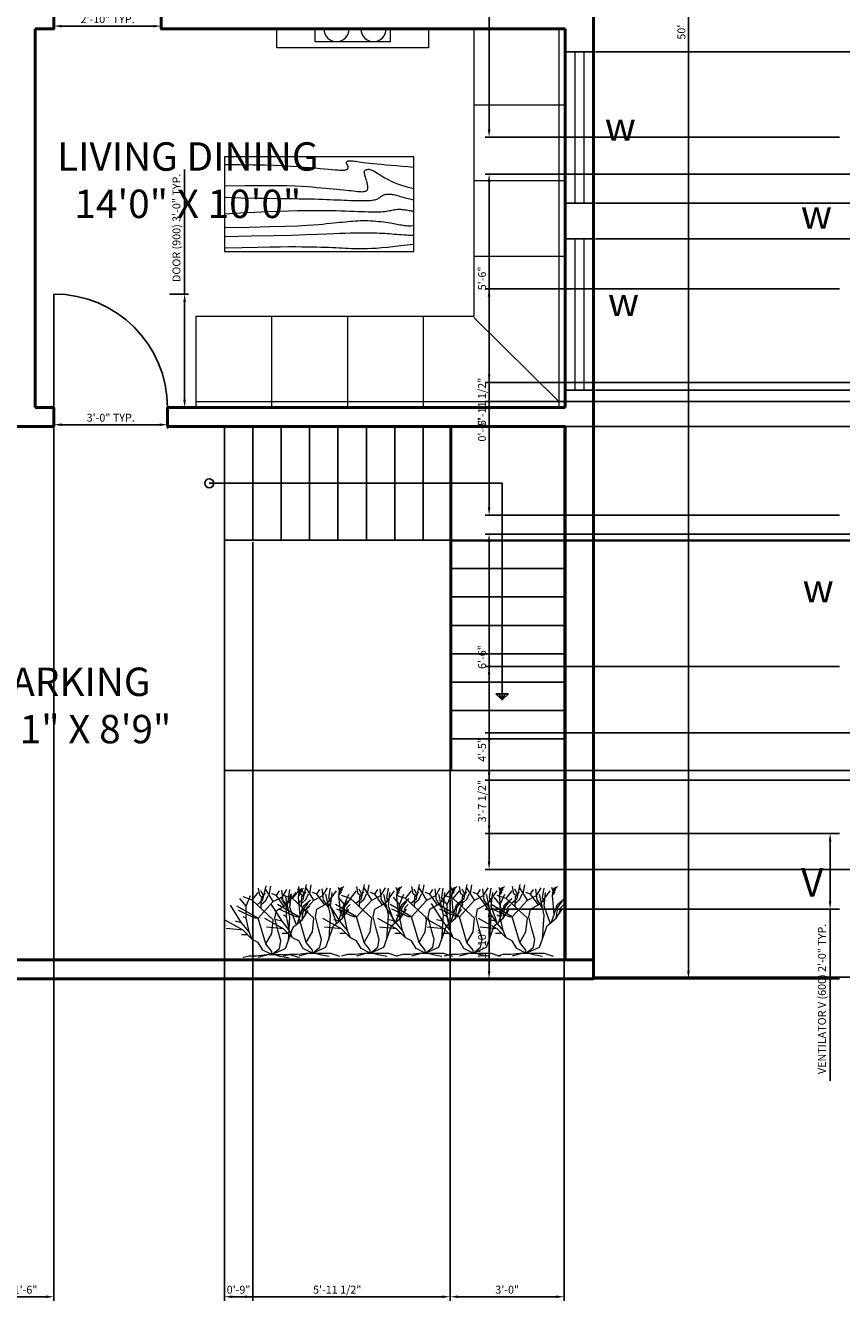
# Model space of a CAD drawing. Units: inches. Extents: x 3688 to 4628, y 1593 to 2337.
# Tile 2 of 7: x 3910 to 4168, y 1593 to 1997. Entities that reach past the tile are written whole.
import ezdxf

# ---------------------------------------------------------------- set-up
doc = ezdxf.new("R2010")
doc.units = ezdxf.units.IN
for name, color, linetype, lineweight in [('A-ANNO-DIMS', 2, 'Continuous', 18), ('A-ANNO-TEXT', 7, 'Continuous', 18), ('A-AREA-IDEN', 7, 'Continuous', 25), ('A-DOOR', 4, 'Continuous', 25), ('A-FLOR-STRS', 3, 'Continuous', 25), ('A-FURN', 8, 'Continuous', 18), ('A-GLAZ', 4, 'Continuous', 25), ('A-WALL', 7, 'Continuous', 50), ('L-PLNT', 3, 'Continuous', 13)]:
    doc.layers.add(name, color=color, linetype=linetype, lineweight=lineweight)
doc.styles.get("Standard").update_dxf_attribs({"font": 'arial.ttf'})
doc.dimstyles.new('ISO-25', dxfattribs={"dimtxt": 2.5, "dimasz": 2.5, "dimexe": 1.25, "dimexo": 0.625, "dimtad": 1, "dimdec": 0, "dimlunit": 3, "dimtxsty": 'Standard', "dimcen": 2.5, "dimadec": 0, "dimazin": 0, "dimtfac": 1, "dimtdec": 0, "dimtmove": 0, "dimatfit": 3, "dimfxl": 1, "dimarcsym": 0})

# ---------------------------------------------------------------- blocks, each defined once
blk = doc.blocks.new('Table - Rectangular Woodgrain 60 x 30 in.')
for p, q in [((0, 0), (0, -30)), ((60, 0), (0, 0)), ((60, -30), (60, 0)), ((0, -30), (60, -30))]:
    blk.add_line(p, q)
for points in [[(0, -2.4), (4.8155, -2.418), (9.0302, -2.4688), (12.709, -2.5477), (15.9167, -2.65), (18.7181, -2.7711), (21.1781, -2.9063), (23.3616, -3.0508), (25.3333, -3.2), (27.1477, -3.3495), (28.8172, -3.4958), (30.3437, -3.636), (31.7291, -3.7667), (32.9756, -3.8849), (34.0849, -3.9875), (35.059, -4.0714), (35.9, -4.1334), (36.6114, -4.1711), (37.2041, -4.1854), (37.6906, -4.1779), (38.0833, -4.15), (38.3948, -4.1034), (38.6375, -4.0396), (38.8239, -3.9602), (38.9666, -3.8667), (39.0764, -3.7608), (39.1573, -3.6448), (39.2116, -3.521), (39.2416, -3.3917), (39.2498, -3.2593), (39.2385, -3.1261), (39.21, -2.9944), (39.1666, -2.8667), (39.111, -2.7447), (39.0468, -2.6281), (38.978, -2.5163), (38.9083, -2.4083), (38.8418, -2.3035), (38.7823, -2.201), (38.7337, -2.1001), (38.7, -2), (38.6844, -1.9003), (38.6875, -1.8021), (38.7094, -1.707), (38.75, -1.6167), (38.8094, -1.5326), (38.8875, -1.4563), (38.9844, -1.3893), (39.1, -1.3333), (39.2351, -1.2896), (39.3937, -1.2583), (39.5804, -1.2396), (39.8, -1.2333), (40.057, -1.2396), (40.3562, -1.2583), (40.7023, -1.2896), (41.1, -1.3333), (41.5547, -1.3895), (42.0755, -1.4573), (42.6721, -1.5361), (43.3542, -1.625), (44.1316, -1.7233), (45.014, -1.8302), (46.0114, -1.9449), (47.1333, -2.0667), (48.3862, -2.1947), (49.7625, -2.3281), (51.2513, -2.4663), (52.8416, -2.6083), (54.5226, -2.7535), (56.2833, -2.9011), (58.1127, -3.0501), (60, -3.2)], [(0, -9.2), (6.5759, -9.0858), (11.9385, -9.0365), (16.2527, -9.0418), (19.6833, -9.0917), (22.3952, -9.1759), (24.5531, -9.2844), (26.322, -9.4069), (27.8666, -9.5333), (29.3241, -9.6553), (30.7203, -9.7719), (32.0532, -9.8837), (33.3208, -9.9917), (34.5213, -10.0965), (35.6526, -10.199), (36.7128, -10.2999), (37.7, -10.4), (38.6129, -10.4996), (39.4531, -10.5969), (40.223, -10.6895), (40.925, -10.775), (41.5613, -10.8512), (42.1344, -10.9156), (42.6465, -10.966), (43.1, -11), (43.4976, -11.0158), (43.8437, -11.0136), (44.143, -10.9942), (44.4, -10.9583), (44.6195, -10.9069), (44.8062, -10.8406), (44.9648, -10.7603), (45.1, -10.6667), (45.2155, -10.5598), (45.3114, -10.4365), (45.3871, -10.2929), (45.4416, -10.125), (45.4743, -9.929), (45.4844, -9.7011), (45.4709, -9.4371), (45.4333, -9.1333), (45.3716, -8.7883), (45.2896, -8.4104), (45.1919, -8.0107), (45.0833, -7.6), (44.9685, -7.1893), (44.8521, -6.7896), (44.7388, -6.4117), (44.6333, -6.0667), (44.54, -5.7628), (44.4614, -5.4979), (44.4001, -5.2675), (44.3583, -5.0667), (44.3384, -4.8909), (44.3427, -4.7354), (44.3736, -4.5956), (44.4333, -4.4667), (44.5236, -4.3453), (44.6427, -4.2333), (44.7884, -4.1339), (44.9583, -4.05), (45.1501, -3.9849), (45.3614, -3.9417), (45.59, -3.9234), (45.8333, -3.9333), (46.0915, -3.9749), (46.3734, -4.0531), (46.6906, -4.1736), (47.0542, -4.3417), (47.4756, -4.5629), (47.9661, -4.8427), (48.5372, -5.1866), (49.2, -5.6), (49.9676, -6.0844), (50.8594, -6.625), (51.8965, -7.2031), (53.1, -7.8), (54.491, -8.3969), (56.0906, -8.975), (57.9199, -9.5156), (60, -10)], [(0, -12.8), (5.1847, -12.9322), (9.6213, -13.0323), (13.3963, -13.1059), (16.5958, -13.1583), (19.3063, -13.1952), (21.614, -13.2219), (23.6054, -13.2439), (25.3666, -13.2667), (26.9728, -13.2947), (28.4531, -13.3281), (29.8256, -13.3663), (31.1083, -13.4083), (32.3191, -13.4535), (33.476, -13.501), (34.597, -13.5501), (35.7, -13.6), (36.7984, -13.6497), (37.8875, -13.6979), (38.9578, -13.743), (40, -13.7833), (41.0047, -13.8174), (41.9625, -13.8438), (42.864, -13.8607), (43.7, -13.8667), (44.4631, -13.8604), (45.1552, -13.8417), (45.7801, -13.8104), (46.3416, -13.7667), (46.8439, -13.7104), (47.2906, -13.6417), (47.6858, -13.5604), (48.0333, -13.4667), (48.3375, -13.3608), (48.6042, -13.2448), (48.8396, -13.121), (49.05, -12.9917), (49.2417, -12.8593), (49.4208, -12.7261), (49.5937, -12.5944), (49.7667, -12.4667), (49.9452, -12.3451), (50.1323, -12.2313), (50.3303, -12.1268), (50.5416, -12.0333), (50.7686, -11.9524), (51.0135, -11.8854), (51.2788, -11.8341), (51.5666, -11.8), (51.8785, -11.7843), (52.2116, -11.7865), (52.562, -11.8059), (52.926, -11.8417), (53.2998, -11.8931), (53.6795, -11.9594), (54.0614, -12.0397), (54.4416, -12.1333), (54.8223, -12.2401), (55.2293, -12.3625), (55.6942, -12.5037), (56.2489, -12.6667), (56.9251, -12.8547), (57.7545, -13.0708), (58.7689, -13.3182), (60, -13.6)], [(0, -18), (5.124, -17.7273), (9.6609, -17.5057), (13.6705, -17.3303), (17.2125, -17.1958), (20.3467, -17.0973), (23.1328, -17.0297), (25.6307, -16.9878), (27.9, -16.9667), (29.9928, -16.9617), (31.9302, -16.9703), (33.7254, -16.9907), (35.3917, -17.0208), (36.9423, -17.0588), (38.3906, -17.1026), (39.7499, -17.1503), (41.0333, -17.2), (42.2519, -17.2496), (43.4073, -17.2969), (44.4986, -17.3395), (45.525, -17.375), (46.4858, -17.4012), (47.3802, -17.4156), (48.2074, -17.416), (48.9667, -17.4), (49.6583, -17.3662), (50.2872, -17.3167), (50.8595, -17.2547), (51.3812, -17.1833), (51.8584, -17.1057), (52.2971, -17.025), (52.7034, -16.9443), (53.0833, -16.8667), (53.443, -16.7951), (53.789, -16.7313), (54.128, -16.6768), (54.4666, -16.6334), (54.8115, -16.6024), (55.1693, -16.5854), (55.5465, -16.5841), (55.95, -16.6), (56.3828, -16.6337), (56.8346, -16.6823), (57.2915, -16.7418), (57.7396, -16.8084), (58.165, -16.878), (58.5539, -16.9469), (58.8924, -17.0111), (59.1666, -17.0667), (59.3679, -17.1107), (59.5078, -17.1438), (59.6032, -17.1675), (59.6708, -17.1833), (59.7275, -17.193), (59.7901, -17.1979), (59.8753, -17.1998), (60, -17.2)], [(0, -22.4), (8.0098, -22.2501), (14.4094, -22.1011), (19.4168, -21.9535), (23.25, -21.8083), (26.1269, -21.6663), (28.2656, -21.5281), (29.884, -21.3947), (31.2, -21.2667), (32.3967, -21.1448), (33.5172, -21.0292), (34.5697, -20.9198), (35.5625, -20.8167), (36.5037, -20.7198), (37.4015, -20.6292), (38.2642, -20.5448), (39.1, -20.4667), (39.9164, -20.3951), (40.7187, -20.3313), (41.5117, -20.2768), (42.3, -20.2333), (43.0883, -20.2024), (43.8812, -20.1854), (44.6836, -20.1841), (45.5, -20.2), (46.3328, -20.234), (47.1747, -20.2844), (48.0163, -20.3488), (48.8479, -20.425), (49.66, -20.5106), (50.4429, -20.6031), (51.1872, -20.7004), (51.8833, -20.8), (52.5246, -20.8999), (53.1166, -20.9995), (53.6681, -21.0983), (54.1875, -21.1958), (54.6834, -21.2919), (55.1646, -21.3859), (55.6394, -21.4777), (56.1167, -21.5667), (56.6028, -21.6515), (57.0961, -21.7266), (57.5929, -21.7852), (58.0896, -21.8208), (58.5823, -21.8268), (59.0674, -21.7964), (59.5412, -21.723), (60, -21.6)], [(0, -25.2), (8.6355, -25.0504), (15.7026, -24.9031), (21.4049, -24.7606), (25.9458, -24.625), (29.529, -24.4988), (32.3578, -24.3844), (34.6359, -24.284), (36.5667, -24.2), (38.3213, -24.1341), (39.9417, -24.0854), (41.437, -24.0523), (42.8167, -24.0333), (44.0901, -24.0268), (45.2667, -24.0313), (46.3557, -24.0451), (47.3667, -24.0667), (48.309, -24.0947), (49.1928, -24.1287), (50.0284, -24.168), (50.826, -24.2125), (51.5959, -24.2617), (52.3483, -24.3151), (53.0935, -24.3725), (53.8417, -24.4334), (54.6009, -24.497), (55.3699, -24.561), (56.1454, -24.6226), (56.9239, -24.6792), (57.7021, -24.7279), (58.4764, -24.7662), (59.2435, -24.7911), (60, -24.8)], [(0, -28.8), (5.6867, -28.6681), (10.45, -28.5698), (14.407, -28.5012), (17.675, -28.4584), (20.3711, -28.4374), (22.6125, -28.4344), (24.5164, -28.4455), (26.2, -28.4667), (27.762, -28.4947), (29.2276, -28.5281), (30.6033, -28.5663), (31.8958, -28.6084), (33.1118, -28.6535), (34.2578, -28.7011), (35.3405, -28.7501), (36.3666, -28.8), (37.3443, -28.8497), (38.288, -28.8974), (39.2137, -28.9412), (40.1375, -28.9792), (41.0753, -29.0093), (42.0432, -29.0297), (43.0572, -29.0384), (44.1333, -29.0333), (45.2936, -29.0114), (46.5843, -28.9641), (48.0579, -28.8816), (49.7666, -28.7542), (51.7629, -28.5721), (54.0989, -28.3255), (56.8272, -28.0048), (60, -27.6)]]:
    blk.add_lwpolyline(points)
blk = doc.blocks.new('*U12')
for p, q in [((-14.88, 18.24), (-12.96, 20.64)), ((-12.471, 19.775), (-12.898, 22.044)), ((-11.28, 19.619), (-12.104, 21.184)), ((-11.921, 18.836), (-10.64, 20.401)), ((-11.433, 18.289), (-10.457, 22.749)), ((-8.16, 17.76), (-10.56, 21.6)), ((-9.48, 19.775), (-8.992, 22.592)), ((-7.2, 19.68), (-6.24, 21.12)), ((-5.086, 17.741), (-5.513, 21.34)), ((-5.28, 19.2), (-3.84, 21.6)), ((-3.84, 16.8), (-0.96, 20.64)), ((-3.377, 18.602), (-2.888, 21.575)), ((-0.508, 21.888), (-0.081, 20.558)), ((-0.203, 19.149), (0.102, 21.34)), ((-0.142, 19.384), (0.59, 20.401)), ((-0.02, 20.01), (0.896, 21.105)), ((0.041, 20.714), (1.384, 22.044)), ((0.102, 21.34), (0.835, 21.888)), ((-18.24, 11.04), (-21.755, 16.655)), ((-12.96, 12.48), (-19.68, 16.32)), ((-16.8, 16.32), (-18.72, 18.72)), ((-14.88, 18.24), (-17.76, 19.2)), ((-16.8, 16.32), (-15.36, 19.68)), ((-16.8, 12.48), (-16.8, 16.32)), ((-8.16, 12), (-14.88, 18.24)), ((-13.325, 16.724), (-11.433, 18.289)), ((-12.96, 12.48), (-8.16, 17.76)), ((-11.677, 19.071), (-12.471, 19.775)), ((-12.043, 15.628), (-11.921, 18.836)), ((-11.982, 16.802), (-10.579, 18.054)), ((-10.579, 18.054), (-9.846, 19.697)), ((-7.2, 19.68), (-8.64, 20.16)), ((-8.16, 17.76), (-5.28, 19.2)), ((-4.8, 16.32), (-7.2, 19.68)), ((-7.2, 14.88), (-3.84, 16.8)), ((-3.377, 15.315), (-5.086, 17.819)), ((-2.88, 12.96), (-4.32, 19.68)), ((-2.766, 16.802), (-3.377, 18.602)), ((-2.88, 15.84), (-2.4, 20.16)), ((0.346, 13.203), (-0.203, 19.149)), ((0.346, 13.203), (1.323, 16.254)), ((1.323, 16.254), (3.642, 18.289)), ((1.44, 15.36), (2.88, 17.28)), ((2.4, 15.36), (3.36, 16.32)), ((-13.92, 12.48), (-19.2, 14.88)), ((-16.8, 12.48), (-17.76, 12.96)), ((-15.84, 8.16), (-16.8, 12.48)), ((-12.96, 12.48), (-13.92, 12.48)), ((-10.56, 4.32), (-12.96, 12.48)), ((-7.68, 12.48), (-7.2, 14.88)), ((-6.72, 8.64), (-7.68, 12.48)), ((-3.36, 5.28), (-2.88, 12.96)), ((-0.96, 10.56), (-2.88, 15.84)), ((-0.48, 10.8), (0.346, 13.203)), ((0.96, 12), (1.44, 15.36)), ((0.96, 12), (2.88, 14.88)), ((1.92, 13.44), (2.4, 15.36)), ((-17.76, 8.64), (-23.663, 11.961)), ((-17.76, 8.64), (-23.128, 9.222)), ((-18.24, 11.04), (-20.16, 11.52)), ((-15.84, 8.16), (-18.24, 11.04)), ((-14.88, 5.76), (-17.76, 8.64)), ((-14.88, 5.76), (-15.84, 8.16)), ((-8.64, 7.68), (-8.16, 12)), ((-5.76, 5.28), (-6.72, 8.64)), ((-4.32, 2.88), (-1.92, 9.6)), ((-1.92, 9.6), (0.96, 12)), ((-16.32, 7.2), (-18.24, 7.2)), ((-12.96, 4.8), (-14.88, 5.76)), ((-11.52, 2.4), (-12.96, 4.8)), ((-10.56, 4.32), (-8.64, 7.68)), ((-8.64, 1.92), (-10.56, 4.32)), ((-6.24, 2.88), (-5.76, 5.28)), ((-15.84, 0.48), (-17.76, 0)), ((-13.44, 0.48), (-15.84, 0.48)), ((-9.6, 0.96), (-13.44, 0.48)), ((-9.6, 0.96), (-12.96, 0)), ((-8.64, 0.96), (-11.52, 2.4)), ((-9.6, 0.96), (-7.68, 0.96)), ((-8.64, 0.96), (-4.32, 2.88)), ((-8.64, 0.96), (-6.24, 2.88)), ((-8.64, 0.96), (-8.64, 1.92)), ((-8.64, 0.96), (-2.88, 0.96)), ((-7.68, 0.96), (-6.24, 0.48)), ((-6.24, 0.48), (-3.36, 0)), ((-2.88, 0.96), (0, 0))]:
    blk.add_line(p, q)
blk = doc.blocks.new('*D17')
at = {"layer": 'A-ANNO-DIMS', "color": 0, "lineweight": -2, "transparency": 16777216}
for p, q in [((4090.25, 2295.32), (4120.92, 2295.32)), ((4119.67, 2292.82), (4119.67, 1697.82)), ((4090.25, 1695.32), (4120.92, 1695.32))]:
    blk.add_line(p, q, dxfattribs=at)
at = {"layer": 'A-ANNO-DIMS', "color": 0, "transparency": 16777216}
for points in [[(4119.25, 2292.82), (4120.08, 2292.82), (4119.67, 2295.32)], [(4119.25, 1697.82), (4120.08, 1697.82), (4119.67, 1695.32)]]:
    blk.add_solid(points, dxfattribs=at)
at = {"layer": 'Defpoints', "color": 0, "transparency": 16777216}
for p in [(4089.62, 2295.32), (4089.62, 1695.32), (4119.67, 1695.32)]:
    blk.add_point(p, dxfattribs=at)
at = {"layer": 'A-ANNO-DIMS', "color": 0, "transparency": 16777216, "insert": (4117.76, 1995.32), "char_height": 2.5, "attachment_point": 5, "rotation": 90}
blk.add_mtext("50'", dxfattribs=at)
blk = doc.blocks.new('DOOR-900')
blk.add_line((0, 0), (0, 36))
blk.add_arc((0, 0), 36, 0, 90)
blk = doc.blocks.new('WIN-1200')
for p, q in [((0, 48), (0, 0)), ((9, 48), (0, 48)), ((9, 0), (9, 48)), ((0, 0), (9, 0))]:
    blk.add_line(p, q)
blk = doc.blocks.new('*D25')
at = {"layer": 'A-ANNO-DIMS', "color": 0, "lineweight": -2, "transparency": 16777216}
for p, q in [((4167.51, 1741.42), (4163.28, 1741.42)), ((4164.53, 1738.92), (4164.53, 1719.92)), ((4167.51, 1717.42), (4163.28, 1717.42)), ((4164.53, 1717.42), (4164.53, 1662.98))]:
    blk.add_line(p, q, dxfattribs=at)
at = {"layer": 'A-ANNO-DIMS', "color": 0, "transparency": 16777216}
for points in [[(4164.12, 1738.92), (4164.95, 1738.92), (4164.53, 1741.42)], [(4164.12, 1719.92), (4164.95, 1719.92), (4164.53, 1717.42)]]:
    blk.add_solid(points, dxfattribs=at)
at = {"layer": 'Defpoints', "color": 0, "transparency": 16777216}
for p in [(4168.13, 1741.42), (4164.53, 1717.42), (4168.13, 1717.42)]:
    blk.add_point(p, dxfattribs=at)
at = {"layer": 'A-ANNO-DIMS', "color": 0, "transparency": 16777216, "insert": (4162.27, 1688.95), "char_height": 2.5, "attachment_point": 5, "rotation": 90}
blk.add_mtext('VENTILATOR V (600) 2\'-0" TYP.', dxfattribs=at)
blk = doc.blocks.new('*D27')
at = {"layer": 'A-ANNO-DIMS', "color": 0, "lineweight": -2, "transparency": 16777216}
for p, q in [((3960.02, 1912.32), (3960.02, 1951.76)), ((3955.25, 1912.32), (3961.27, 1912.32)), ((3960.02, 1878.82), (3960.02, 1909.82)), ((3955.25, 1876.32), (3961.27, 1876.32))]:
    blk.add_line(p, q, dxfattribs=at)
at = {"layer": 'A-ANNO-DIMS', "color": 0, "transparency": 16777216}
for points in [[(3959.61, 1909.82), (3960.44, 1909.82), (3960.02, 1912.32)], [(3959.61, 1878.82), (3960.44, 1878.82), (3960.02, 1876.32)]]:
    blk.add_solid(points, dxfattribs=at)
at = {"layer": 'Defpoints', "color": 0, "transparency": 16777216}
for p in [(3954.62, 1912.32), (3960.02, 1912.32), (3954.62, 1876.32)]:
    blk.add_point(p, dxfattribs=at)
at = {"layer": 'A-ANNO-DIMS', "color": 0, "transparency": 16777216, "insert": (3957.76, 1933.29), "char_height": 2.5, "attachment_point": 5, "rotation": 90}
blk.add_mtext('DOOR (900) 3\'-0" TYP.', dxfattribs=at)
blk = doc.blocks.new('*D28')
at = {"layer": 'A-ANNO-DIMS', "color": 0, "lineweight": -2, "transparency": 16777216}
for p, q in [((3918.62, 1875.69), (3918.62, 1869.67)), ((3954.62, 1875.69), (3954.62, 1869.67)), ((3921.12, 1870.92), (3952.12, 1870.92))]:
    blk.add_line(p, q, dxfattribs=at)
at = {"layer": 'A-ANNO-DIMS', "color": 0, "transparency": 16777216}
for points in [[(3921.12, 1871.34), (3921.12, 1870.5), (3918.62, 1870.92)], [(3952.12, 1871.34), (3952.12, 1870.5), (3954.62, 1870.92)]]:
    blk.add_solid(points, dxfattribs=at)
at = {"layer": 'Defpoints', "color": 0, "transparency": 16777216}
for p in [(3918.62, 1876.32), (3954.62, 1876.32), (3954.62, 1870.92)]:
    blk.add_point(p, dxfattribs=at)
at = {"layer": 'A-ANNO-DIMS', "color": 0, "transparency": 16777216, "insert": (3936.62, 1872.82), "char_height": 2.5, "attachment_point": 5}
blk.add_mtext('3\'-0" TYP.', dxfattribs=at)
blk = doc.blocks.new('*D30')
at = {"layer": 'A-ANNO-DIMS', "color": 0, "lineweight": -2, "transparency": 16777216}
for p, q in [((3918.62, 2001.69), (3918.62, 1995.97)), ((3952.62, 2001.69), (3952.62, 1995.97)), ((3921.12, 1997.22), (3950.12, 1997.22))]:
    blk.add_line(p, q, dxfattribs=at)
at = {"layer": 'A-ANNO-DIMS', "color": 0, "transparency": 16777216}
for points in [[(3921.12, 1997.64), (3921.12, 1996.8), (3918.62, 1997.22)], [(3950.12, 1997.64), (3950.12, 1996.8), (3952.62, 1997.22)]]:
    blk.add_solid(points, dxfattribs=at)
at = {"layer": 'Defpoints', "color": 0, "transparency": 16777216}
for p in [(3918.62, 2002.32), (3952.62, 2002.32), (3952.62, 1997.22)]:
    blk.add_point(p, dxfattribs=at)
at = {"layer": 'A-ANNO-DIMS', "color": 0, "transparency": 16777216, "insert": (3935.62, 1999.12), "char_height": 2.5, "attachment_point": 5}
blk.add_mtext('2\'-10" TYP.', dxfattribs=at)
blk = doc.blocks.new('*D59')
at = {"layer": 'A-ANNO-DIMS', "color": 0, "lineweight": -2, "transparency": 16777216}
for p, q in [((4090.25, 2025.17), (4188.4, 2025.17)), ((4187.15, 2022.67), (4187.15, 1991.6)), ((4090.25, 1989.1), (4188.4, 1989.1))]:
    blk.add_line(p, q, dxfattribs=at)
at = {"layer": 'A-ANNO-DIMS', "color": 0, "transparency": 16777216}
for points in [[(4186.74, 2022.67), (4187.57, 2022.67), (4187.15, 2025.17)], [(4186.74, 1991.6), (4187.57, 1991.6), (4187.15, 1989.1)]]:
    blk.add_solid(points, dxfattribs=at)
at = {"layer": 'Defpoints', "color": 0, "transparency": 16777216}
for p in [(4089.62, 2025.17), (4089.62, 1989.1), (4187.15, 1989.1)]:
    blk.add_point(p, dxfattribs=at)
at = {"layer": 'A-ANNO-DIMS', "color": 0, "transparency": 16777216, "insert": (4185.25, 2007.14), "char_height": 2.5, "attachment_point": 5, "rotation": 90}
blk.add_mtext('3\'-0"', dxfattribs=at)
blk = doc.blocks.new('*D60')
at = {"layer": 'A-ANNO-DIMS', "color": 0, "lineweight": -2, "transparency": 16777216}
for p, q in [((4090.25, 1941.1), (4188.4, 1941.1)), ((4187.15, 1938.6), (4187.15, 1932.34)), ((4090.25, 1929.84), (4188.4, 1929.84)), ((4187.15, 1929.84), (4187.15, 1911.67))]:
    blk.add_line(p, q, dxfattribs=at)
at = {"layer": 'A-ANNO-DIMS', "color": 0, "transparency": 16777216}
for points in [[(4186.74, 1938.6), (4187.57, 1938.6), (4187.15, 1941.1)], [(4186.74, 1932.34), (4187.57, 1932.34), (4187.15, 1929.84)]]:
    blk.add_solid(points, dxfattribs=at)
at = {"layer": 'Defpoints', "color": 0, "transparency": 16777216}
for p in [(4089.62, 1941.1), (4089.62, 1929.84), (4187.15, 1929.84)]:
    blk.add_point(p, dxfattribs=at)
at = {"layer": 'A-ANNO-DIMS', "color": 0, "transparency": 16777216, "insert": (4185.24, 1919.5), "char_height": 2.5, "attachment_point": 5, "rotation": 90}
blk.add_mtext('0\'-11 1/2"', dxfattribs=at)
blk = doc.blocks.new('*D61')
at = {"layer": 'A-ANNO-DIMS', "color": 0, "lineweight": -2, "transparency": 16777216}
for p, q in [((4090.25, 1881.84), (4188.4, 1881.84)), ((4187.15, 1879.34), (4187.15, 1698.33)), ((4090.03, 1695.83), (4188.4, 1695.83))]:
    blk.add_line(p, q, dxfattribs=at)
at = {"layer": 'A-ANNO-DIMS', "color": 0, "transparency": 16777216}
for points in [[(4186.74, 1879.34), (4187.57, 1879.34), (4187.15, 1881.84)], [(4186.74, 1698.33), (4187.57, 1698.33), (4187.15, 1695.83)]]:
    blk.add_solid(points, dxfattribs=at)
at = {"layer": 'Defpoints', "color": 0, "transparency": 16777216}
for p in [(4089.62, 1881.84), (4089.41, 1695.83), (4187.15, 1695.83)]:
    blk.add_point(p, dxfattribs=at)
at = {"layer": 'A-ANNO-DIMS', "color": 0, "transparency": 16777216, "insert": (4185.25, 1788.83), "char_height": 2.5, "attachment_point": 5, "rotation": 90}
blk.add_mtext('15\'-6"', dxfattribs=at)
blk = doc.blocks.new('*D72')
at = {"layer": 'A-ANNO-DIMS', "color": 0, "lineweight": -2, "transparency": 16777216}
for p, q in [((3900.62, 1869.69), (3900.62, 1593.32)), ((3918.62, 1869.69), (3918.62, 1593.32)), ((3903.12, 1594.57), (3916.12, 1594.57))]:
    blk.add_line(p, q, dxfattribs=at)
at = {"layer": 'A-ANNO-DIMS', "color": 0, "transparency": 16777216}
for points in [[(3903.12, 1594.98), (3903.12, 1594.15), (3900.62, 1594.57)], [(3916.12, 1594.98), (3916.12, 1594.15), (3918.62, 1594.57)]]:
    blk.add_solid(points, dxfattribs=at)
at = {"layer": 'Defpoints', "color": 0, "transparency": 16777216}
for p in [(3900.62, 1870.32), (3918.62, 1870.32), (3918.62, 1594.57)]:
    blk.add_point(p, dxfattribs=at)
at = {"layer": 'A-ANNO-DIMS', "color": 0, "transparency": 16777216, "insert": (3909.62, 1596.47), "char_height": 2.5, "attachment_point": 5}
blk.add_mtext('1\'-6"', dxfattribs=at)
blk = doc.blocks.new('*D75')
at = {"layer": 'A-ANNO-DIMS', "color": 0, "lineweight": -2, "transparency": 16777216}
for p, q in [((3972.62, 1869.69), (3972.62, 1593.32)), ((4044.16, 1869.84), (4044.16, 1593.32)), ((3975.12, 1594.57), (4041.66, 1594.57))]:
    blk.add_line(p, q, dxfattribs=at)
at = {"layer": 'A-ANNO-DIMS', "color": 0, "transparency": 16777216}
for points in [[(3975.12, 1594.98), (3975.12, 1594.15), (3972.62, 1594.57)], [(4041.66, 1594.98), (4041.66, 1594.15), (4044.16, 1594.57)]]:
    blk.add_solid(points, dxfattribs=at)
at = {"layer": 'Defpoints', "color": 0, "transparency": 16777216}
for p in [(3972.62, 1870.32), (4044.16, 1870.47), (4044.16, 1594.57)]:
    blk.add_point(p, dxfattribs=at)
at = {"layer": 'A-ANNO-DIMS', "color": 0, "transparency": 16777216, "insert": (4008.39, 1596.48), "char_height": 2.5, "attachment_point": 5}
blk.add_mtext('5\'-11 1/2"', dxfattribs=at)
blk = doc.blocks.new('*D76')
at = {"layer": 'A-ANNO-DIMS', "color": 0, "lineweight": -2, "transparency": 16777216}
for p, q in [((4044.16, 1869.84), (4044.16, 1593.32)), ((4080.3, 1869.59), (4080.3, 1593.32)), ((4046.66, 1594.57), (4077.8, 1594.57))]:
    blk.add_line(p, q, dxfattribs=at)
at = {"layer": 'A-ANNO-DIMS', "color": 0, "transparency": 16777216}
for points in [[(4046.66, 1594.98), (4046.66, 1594.15), (4044.16, 1594.57)], [(4077.8, 1594.98), (4077.8, 1594.15), (4080.3, 1594.57)]]:
    blk.add_solid(points, dxfattribs=at)
at = {"layer": 'Defpoints', "color": 0, "transparency": 16777216}
for p in [(4044.16, 1870.47), (4080.3, 1870.22), (4080.3, 1594.57)]:
    blk.add_point(p, dxfattribs=at)
at = {"layer": 'A-ANNO-DIMS', "color": 0, "transparency": 16777216, "insert": (4062.23, 1596.47), "char_height": 2.5, "attachment_point": 5}
blk.add_mtext('3\'-0"', dxfattribs=at)
blk = doc.blocks.new('*D77')
at = {"layer": 'A-ANNO-DIMS', "color": 0, "lineweight": -2, "transparency": 16777216}
for p, q in [((3972.62, 1833.69), (3972.62, 1593.32)), ((3981.62, 1833.69), (3981.62, 1593.32)), ((3975.12, 1594.57), (3979.12, 1594.57))]:
    blk.add_line(p, q, dxfattribs=at)
at = {"layer": 'A-ANNO-DIMS', "color": 0, "transparency": 16777216}
for points in [[(3975.12, 1594.98), (3975.12, 1594.15), (3972.62, 1594.57)], [(3979.12, 1594.98), (3979.12, 1594.15), (3981.62, 1594.57)]]:
    blk.add_solid(points, dxfattribs=at)
at = {"layer": 'Defpoints', "color": 0, "transparency": 16777216}
for p in [(3972.62, 1834.32), (3981.62, 1834.32), (3981.62, 1594.57)]:
    blk.add_point(p, dxfattribs=at)
at = {"layer": 'A-ANNO-DIMS', "color": 0, "transparency": 16777216, "insert": (3977.12, 1596.47), "char_height": 2.5, "attachment_point": 5}
blk.add_mtext('0\'-9"', dxfattribs=at)
blk = doc.blocks.new('*D78')
at = {"layer": 'A-ANNO-DIMS', "color": 0, "lineweight": -2, "transparency": 16777216}
for p, q in [((3973.25, 1870.32), (4188.4, 1870.32)), ((4187.15, 1867.82), (4187.15, 1836.82)), ((3973.25, 1834.32), (4188.4, 1834.32))]:
    blk.add_line(p, q, dxfattribs=at)
at = {"layer": 'A-ANNO-DIMS', "color": 0, "transparency": 16777216}
for points in [[(4186.74, 1867.82), (4187.57, 1867.82), (4187.15, 1870.32)], [(4186.74, 1836.82), (4187.57, 1836.82), (4187.15, 1834.32)]]:
    blk.add_solid(points, dxfattribs=at)
at = {"layer": 'Defpoints', "color": 0, "transparency": 16777216}
for p in [(3972.62, 1870.32), (3972.62, 1834.32), (4187.15, 1834.32)]:
    blk.add_point(p, dxfattribs=at)
at = {"layer": 'A-ANNO-DIMS', "color": 0, "transparency": 16777216, "insert": (4185.25, 1852.32), "char_height": 2.5, "attachment_point": 5, "rotation": 90}
blk.add_mtext('3\'-0"', dxfattribs=at)
blk = doc.blocks.new('*D79')
at = {"layer": 'A-ANNO-DIMS', "color": 0, "lineweight": -2, "transparency": 16777216}
for p, q in [((4044.44, 1834.15), (4188.4, 1834.15)), ((4187.15, 1831.65), (4187.15, 1763.82)), ((4045.25, 1761.32), (4188.4, 1761.32))]:
    blk.add_line(p, q, dxfattribs=at)
at = {"layer": 'A-ANNO-DIMS', "color": 0, "transparency": 16777216}
for points in [[(4186.74, 1831.65), (4187.57, 1831.65), (4187.15, 1834.15)], [(4186.74, 1763.82), (4187.57, 1763.82), (4187.15, 1761.32)]]:
    blk.add_solid(points, dxfattribs=at)
at = {"layer": 'Defpoints', "color": 0, "transparency": 16777216}
for p in [(4043.81, 1834.15), (4044.62, 1761.32), (4187.15, 1761.32)]:
    blk.add_point(p, dxfattribs=at)
at = {"layer": 'A-ANNO-DIMS', "color": 0, "transparency": 16777216, "insert": (4185.25, 1797.73), "char_height": 2.5, "attachment_point": 5, "rotation": 90}
blk.add_mtext('6\'-1"', dxfattribs=at)
blk = doc.blocks.new('*D81')
at = {"layer": 'A-ANNO-DIMS', "color": 0, "lineweight": -2, "transparency": 16777216}
for p, q in [((4167.51, 2138.96), (4055.24, 2138.96)), ((4056.49, 2136.46), (4056.49, 1964.52)), ((4167.51, 1962.02), (4055.24, 1962.02))]:
    blk.add_line(p, q, dxfattribs=at)
at = {"layer": 'A-ANNO-DIMS', "color": 0, "transparency": 16777216}
for points in [[(4056.07, 2136.46), (4056.9, 2136.46), (4056.49, 2138.96)], [(4056.07, 1964.52), (4056.9, 1964.52), (4056.49, 1962.02)]]:
    blk.add_solid(points, dxfattribs=at)
at = {"layer": 'Defpoints', "color": 0, "transparency": 16777216}
for p in [(4168.13, 2138.96), (4056.49, 1962.02), (4168.13, 1962.02)]:
    blk.add_point(p, dxfattribs=at)
at = {"layer": 'A-ANNO-DIMS', "color": 0, "transparency": 16777216, "insert": (4054.58, 2050.49), "char_height": 2.5, "attachment_point": 5, "rotation": 90}
blk.add_mtext('14\'-9"', dxfattribs=at)
blk = doc.blocks.new('*D82')
at = {"layer": 'A-ANNO-DIMS', "color": 0, "lineweight": -2, "transparency": 16777216}
for p, q in [((4167.51, 1914.02), (4055.24, 1914.02)), ((4056.49, 1911.52), (4056.49, 1844.78)), ((4167.51, 1842.28), (4055.24, 1842.28))]:
    blk.add_line(p, q, dxfattribs=at)
at = {"layer": 'A-ANNO-DIMS', "color": 0, "transparency": 16777216}
for points in [[(4056.07, 1911.52), (4056.9, 1911.52), (4056.49, 1914.02)], [(4056.07, 1844.78), (4056.9, 1844.78), (4056.49, 1842.28)]]:
    blk.add_solid(points, dxfattribs=at)
at = {"layer": 'Defpoints', "color": 0, "transparency": 16777216}
for p in [(4168.13, 1914.02), (4056.49, 1842.28), (4168.13, 1842.28)]:
    blk.add_point(p, dxfattribs=at)
at = {"layer": 'A-ANNO-DIMS', "color": 0, "transparency": 16777216, "insert": (4054.57, 1878.15), "char_height": 2.5, "attachment_point": 5, "rotation": 90}
blk.add_mtext('5\'-11 1/2"', dxfattribs=at)
blk = doc.blocks.new('*D83')
at = {"layer": 'A-ANNO-DIMS', "color": 0, "lineweight": -2, "transparency": 16777216}
for p, q in [((4167.51, 1794.28), (4055.24, 1794.28)), ((4056.49, 1791.78), (4056.49, 1743.92)), ((4167.51, 1741.42), (4055.24, 1741.42))]:
    blk.add_line(p, q, dxfattribs=at)
at = {"layer": 'A-ANNO-DIMS', "color": 0, "transparency": 16777216}
for points in [[(4056.07, 1791.78), (4056.9, 1791.78), (4056.49, 1794.28)], [(4056.07, 1743.92), (4056.9, 1743.92), (4056.49, 1741.42)]]:
    blk.add_solid(points, dxfattribs=at)
at = {"layer": 'Defpoints', "color": 0, "transparency": 16777216}
for p in [(4168.13, 1794.28), (4056.49, 1741.42), (4168.13, 1741.42)]:
    blk.add_point(p, dxfattribs=at)
at = {"layer": 'A-ANNO-DIMS', "color": 0, "transparency": 16777216, "insert": (4054.59, 1767.85), "char_height": 2.5, "attachment_point": 5, "rotation": 90}
blk.add_mtext('4\'-5"', dxfattribs=at)
blk = doc.blocks.new('*D84')
at = {"layer": 'A-ANNO-DIMS', "color": 0, "lineweight": -2, "transparency": 16777216}
for p, q in [((4167.51, 1717.42), (4055.24, 1717.42)), ((4056.49, 1714.92), (4056.49, 1697.78)), ((4167.51, 1695.28), (4055.24, 1695.28))]:
    blk.add_line(p, q, dxfattribs=at)
at = {"layer": 'A-ANNO-DIMS', "color": 0, "transparency": 16777216}
for points in [[(4056.07, 1714.92), (4056.9, 1714.92), (4056.49, 1717.42)], [(4056.07, 1697.78), (4056.9, 1697.78), (4056.49, 1695.28)]]:
    blk.add_solid(points, dxfattribs=at)
at = {"layer": 'Defpoints', "color": 0, "transparency": 16777216}
for p in [(4168.13, 1717.42), (4056.49, 1695.28), (4168.13, 1695.28)]:
    blk.add_point(p, dxfattribs=at)
at = {"layer": 'A-ANNO-DIMS', "color": 0, "transparency": 16777216, "insert": (4054.58, 1706.35), "char_height": 2.5, "attachment_point": 5, "rotation": 90}
blk.add_mtext('1\'-10"', dxfattribs=at)
blk = doc.blocks.new('*D99')
at = {"layer": 'A-ANNO-DIMS', "color": 0, "lineweight": -2, "transparency": 16777216}
for p, q in [((4302.51, 1950.28), (4055.24, 1950.28)), ((4056.49, 1947.78), (4056.49, 1886.78)), ((4302.51, 1884.28), (4055.24, 1884.28))]:
    blk.add_line(p, q, dxfattribs=at)
at = {"layer": 'A-ANNO-DIMS', "color": 0, "transparency": 16777216}
for points in [[(4056.07, 1947.78), (4056.9, 1947.78), (4056.49, 1950.28)], [(4056.07, 1886.78), (4056.9, 1886.78), (4056.49, 1884.28)]]:
    blk.add_solid(points, dxfattribs=at)
at = {"layer": 'Defpoints', "color": 0, "transparency": 16777216}
for p in [(4303.13, 1950.28), (4056.49, 1884.28), (4303.13, 1884.28)]:
    blk.add_point(p, dxfattribs=at)
at = {"layer": 'A-ANNO-DIMS', "color": 0, "transparency": 16777216, "insert": (4054.58, 1917.28), "char_height": 2.5, "attachment_point": 5, "rotation": 90}
blk.add_mtext('5\'-6"', dxfattribs=at)
blk = doc.blocks.new('*D101')
at = {"layer": 'A-ANNO-DIMS', "color": 0, "lineweight": -2, "transparency": 16777216}
for p, q in [((4056.49, 1886.78), (4056.49, 1889.28)), ((4296.51, 1884.28), (4055.24, 1884.28)), ((4056.49, 1884.28), (4056.49, 1878.28)), ((4296.51, 1878.28), (4055.24, 1878.28)), ((4056.49, 1875.78), (4056.49, 1865.39))]:
    blk.add_line(p, q, dxfattribs=at)
at = {"layer": 'A-ANNO-DIMS', "color": 0, "transparency": 16777216}
for points in [[(4056.07, 1886.78), (4056.9, 1886.78), (4056.49, 1884.28)], [(4056.07, 1875.78), (4056.9, 1875.78), (4056.49, 1878.28)]]:
    blk.add_solid(points, dxfattribs=at)
at = {"layer": 'Defpoints', "color": 0, "transparency": 16777216}
for p in [(4297.13, 1884.28), (4056.49, 1878.28), (4297.13, 1878.28)]:
    blk.add_point(p, dxfattribs=at)
at = {"layer": 'A-ANNO-DIMS', "color": 0, "transparency": 16777216, "insert": (4054.58, 1869.34), "char_height": 2.5, "attachment_point": 5, "rotation": 90}
blk.add_mtext('0\'-6"', dxfattribs=at)
blk = doc.blocks.new('*D102')
at = {"layer": 'A-ANNO-DIMS', "color": 0, "lineweight": -2, "transparency": 16777216}
for p, q in [((4296.51, 1836.28), (4055.24, 1836.28)), ((4056.49, 1833.78), (4056.49, 1760.78)), ((4296.51, 1758.28), (4055.24, 1758.28))]:
    blk.add_line(p, q, dxfattribs=at)
at = {"layer": 'A-ANNO-DIMS', "color": 0, "transparency": 16777216}
for points in [[(4056.07, 1833.78), (4056.9, 1833.78), (4056.49, 1836.28)], [(4056.07, 1760.78), (4056.9, 1760.78), (4056.49, 1758.28)]]:
    blk.add_solid(points, dxfattribs=at)
at = {"layer": 'Defpoints', "color": 0, "transparency": 16777216}
for p in [(4297.13, 1836.28), (4056.49, 1758.28), (4297.13, 1758.28)]:
    blk.add_point(p, dxfattribs=at)
at = {"layer": 'A-ANNO-DIMS', "color": 0, "transparency": 16777216, "insert": (4054.58, 1797.28), "char_height": 2.5, "attachment_point": 5, "rotation": 90}
blk.add_mtext('6\'-6"', dxfattribs=at)
blk = doc.blocks.new('*D111')
at = {"layer": 'A-ANNO-DIMS', "color": 0, "lineweight": -2, "transparency": 16777216}
for p, q in [((4518.51, 1773.28), (4055.24, 1773.28)), ((4056.49, 1770.78), (4056.49, 1732.46)), ((4516.99, 1729.96), (4055.24, 1729.96))]:
    blk.add_line(p, q, dxfattribs=at)
at = {"layer": 'A-ANNO-DIMS', "color": 0, "transparency": 16777216}
for points in [[(4056.07, 1770.78), (4056.9, 1770.78), (4056.49, 1773.28)], [(4056.07, 1732.46), (4056.9, 1732.46), (4056.49, 1729.96)]]:
    blk.add_solid(points, dxfattribs=at)
at = {"layer": 'Defpoints', "color": 0, "transparency": 16777216}
for p in [(4519.13, 1773.28), (4056.49, 1729.96), (4517.62, 1729.96)]:
    blk.add_point(p, dxfattribs=at)
at = {"layer": 'A-ANNO-DIMS', "color": 0, "transparency": 16777216, "insert": (4054.57, 1751.62), "char_height": 2.5, "attachment_point": 5, "rotation": 90}
blk.add_mtext('3\'-7 1/2"', dxfattribs=at)

msp = doc.modelspace()

# ---------------------------------------------------------------- linework, layer by layer
at = {"layer": 'A-FLOR-STRS'}
for p, q in [((3972.62, 1870.32), (3972.62, 1834.32)), ((3981.62, 1870.32), (3981.62, 1834.32)), ((3990.62, 1870.32), (3990.62, 1834.32)), ((3999.62, 1870.32), (3999.62, 1834.32)), ((4008.62, 1870.32), (4008.62, 1834.32)), ((4017.62, 1870.32), (4017.62, 1834.32)), ((4026.62, 1870.32), (4026.62, 1834.32)), ((4035.62, 1870.32), (4035.62, 1834.32)), ((4044.62, 1870.32), (4044.62, 1761.32)), ((3967.82, 1852.37), (4060.6, 1852.37)), ((4060.6, 1852.37), (4060.6, 1785.68)), ((3972.62, 1834.32), (4080.62, 1834.32)), ((4044.62, 1825.32), (4080.62, 1825.32)), ((4044.62, 1816.32), (4080.62, 1816.32)), ((4044.62, 1807.32), (4080.62, 1807.32)), ((4044.62, 1798.32), (4080.62, 1798.32)), ((4044.62, 1789.32), (4080.62, 1789.32)), ((4060.6, 1785.68), (4058.6, 1785.68)), ((4058.6, 1785.68), (4060.6, 1785.68)), ((4062.6, 1785.68), (4058.6, 1785.68)), ((4058.6, 1785.68), (4060.6, 1783.68)), ((4060.6, 1783.68), (4059.6, 1785.68)), ((4060.6, 1785.68), (4060.6, 1785.68)), ((4060.6, 1785.68), (4062.6, 1785.68)), ((4062.6, 1785.68), (4060.6, 1785.68)), ((4060.6, 1785.68), (4060.6, 1783.68)), ((4060.6, 1783.68), (4062.6, 1785.68)), ((4060.6, 1783.68), (4061.6, 1785.68)), ((4061.6, 1785.68), (4060.6, 1783.68)), ((4044.62, 1780.32), (4080.62, 1780.32)), ((4044.62, 1771.32), (4080.62, 1771.32)), ((3972.62, 1761.32), (3972.62, 1704.32)), ((4080.62, 1761.32), (3972.62, 1761.32)), ((3972.62, 1761.32), (3972.62, 1704.32)), ((3972.69, 1701.32), (3972.62, 1708.22))]:
    msp.add_line(p, q, dxfattribs=at)
msp.add_circle((3967.82, 1852.37), 1.42, dxfattribs=at)
at = {"layer": 'A-FURN'}
for p, q in [((3989.27, 1990.32), (3989.27, 1996.32)), ((3989.27, 1996.32), (4001.27, 1996.32)), ((4001.27, 1996.32), (4001.27, 1992.32)), ((4025.27, 1992.32), (4025.27, 1996.32)), ((4037.27, 1996.32), (4037.27, 1990.32)), ((4051.62, 1996.32), (4051.62, 1905.32)), ((4078.62, 1996.32), (4078.62, 1876.32)), ((4001.27, 1992.32), (4025.27, 1992.32)), ((4037.27, 1990.32), (3989.27, 1990.32)), ((4083.62, 1989.1), (4083.62, 1941.1)), ((4086.62, 1941.1), (4086.62, 1989.1)), ((4051.62, 1972.32), (4080.62, 1972.32)), ((4051.62, 1948.32), (4080.62, 1948.32)), ((4083.62, 1929.84), (4083.62, 1881.84)), ((4086.62, 1881.84), (4086.62, 1929.84)), ((4051.62, 1924.32), (4080.62, 1924.32)), ((3963.58, 1905.32), (4051.62, 1905.32)), ((3963.58, 1905.32), (3963.58, 1876.32)), ((3987.58, 1905.32), (3987.58, 1876.32)), ((4011.58, 1905.32), (4011.58, 1876.32)), ((4035.58, 1905.32), (4035.58, 1876.32)), ((3963.58, 1878.32), (4080.62, 1878.32))]:
    msp.add_line(p, q, dxfattribs=at)
msp.add_lwpolyline([(4051.62, 1904.93), (4078.62, 1878.32)], dxfattribs=at)
for centre, end in [((4008.14, 1996.32), 0), ((4019.87, 1996.32), 360)]:
    msp.add_arc(centre, 4, 180, end, dxfattribs=at)
at = {"layer": 'A-WALL'}
for p, q in [((4089.62, 2295.32), (4089.62, 1695.32)), ((3918.62, 2002.32), (3918.62, 1996.32)), ((3952.62, 1996.32), (3952.62, 2002.32)), ((3912.62, 1996.32), (3912.62, 1876.32)), ((3912.62, 1996.32), (3918.62, 1996.32)), ((3952.62, 1996.32), (4080.62, 1996.32)), ((4080.62, 1996.32), (4080.62, 1876.32)), ((3912.62, 1876.32), (3918.62, 1876.32)), ((3912.62, 1876.32), (3918.62, 1876.32)), ((3918.62, 1876.32), (3918.62, 1870.32)), ((3954.62, 1870.32), (3954.62, 1876.32)), ((3954.62, 1876.32), (4080.62, 1876.32)), ((3900.62, 1870.32), (3918.62, 1870.32)), ((3954.62, 1870.32), (4080.62, 1870.32)), ((4080.62, 1870.32), (4080.62, 1704.32)), ((4080.62, 1704.32), (4080.62, 1701.32)), ((4089.62, 1701.32), (3867.62, 1701.32)), ((4089.62, 1695.32), (3729.62, 1695.32))]:
    msp.add_line(p, q, dxfattribs=at)

# ---------------------------------------------------------------- block references
at = {"layer": 'A-DOOR'}
msp.add_blockref('DOOR-900', (3918.62, 1876.32), dxfattribs=at)
at = {"layer": 'A-FURN'}
msp.add_blockref('Table - Rectangular Woodgrain 60 x 30 in.', (3972.62, 1955.78), dxfattribs=at)
at = {"layer": 'A-GLAZ'}
for p in [(4080.62, 1941.1), (4080.62, 1881.84)]:
    msp.add_blockref('WIN-1200', p, dxfattribs=at)
at = {"layer": 'L-PLNT'}
for p in [(3996.29, 1702.05), (4009.13, 1702.51), (4027.46, 1702.51), (4044.88, 1702.51), (4060.04, 1702.51), (4076.79, 1702.51)]:
    msp.add_blockref('*U12', p, dxfattribs=at)

# ---------------------------------------------------------------- texts
at = {"layer": 'A-ANNO-TEXT', "char_height": 9, "attachment_point": 1}
for s, heights, insert in [('\\pxqc;w', [0], (4028.83, 1969.93)), ('\\pxqc;w', [0], (4090.96, 1942.09)), ('\\pxqc;w', [0], (4029.84, 1914.32)), ('\\pxqc;w', [0], (4091.51, 1823.59)), ('\\pxqc;V', [37.18], (4089.62, 1730.4))]:
    msp.add_mtext_dynamic_manual_height_columns(s, width=138.4723, gutter_width=12.5, heights=heights, dxfattribs=dict(at, insert=insert))
at = {"layer": 'A-AREA-IDEN', "char_height": 9, "attachment_point": 1}
for s, insert in [('\\pxqc;LIVING DINING\\P14\'0" X 10\'0"', (3908.51, 1960.41)), ('\\pxqc;PARKING \\P14\'1" X 8\'9" ', (3870.74, 1793.95))]:
    msp.add_mtext_dynamic_manual_height_columns(s, width=105.0766, gutter_width=12.5, heights=[0], dxfattribs=dict(at, insert=insert))

# ---------------------------------------------------------------- dimensions: what is measured, and where the dimension line sits
at = {"layer": 'A-ANNO-DIMS'}
for base, p1, p2, override, picture, middle in [((4119.67, 1695.32), (4089.62, 2295.32), (4089.62, 1695.32), {"dimclrd": 0, "dimclre": 0, "dimclrt": 0}, '*D17', (4117.76, 1995.32)), ((4056.49, 1962.02), (4168.13, 2138.96), (4168.13, 1962.02), {"dimdec": 1, "dimlfac": 1, "dimrnd": 0, "dimzin": 1, "dimdsep": 46, "dimlunit": 4, "dimfrac": 2}, '*D81', (4054.58, 2050.49)), ((4187.15, 1989.1), (4089.62, 2025.17), (4089.62, 1989.1), {"dimdec": 1, "dimlfac": 1, "dimrnd": 0, "dimzin": 1, "dimdsep": 46, "dimlunit": 4, "dimfrac": 2}, '*D59', (4185.25, 2007.14)), ((4056.49, 1884.28), (4303.13, 1950.28), (4303.13, 1884.28), {"dimdec": 1, "dimlfac": 1, "dimrnd": 0, "dimzin": 1, "dimdsep": 46, "dimlunit": 4, "dimfrac": 2}, '*D99', (4054.58, 1917.28)), ((4187.15, 1929.84), (4089.62, 1941.1), (4089.62, 1929.84), {"dimdec": 1, "dimlfac": 1, "dimrnd": 0, "dimzin": 1, "dimdsep": 46, "dimlunit": 4, "dimfrac": 2}, '*D60', (4185.24, 1919.5)), ((4056.49, 1842.28), (4168.13, 1914.02), (4168.13, 1842.28), {"dimdec": 1, "dimlfac": 1, "dimrnd": 0, "dimzin": 1, "dimdsep": 46, "dimlunit": 4, "dimfrac": 2}, '*D82', (4054.57, 1878.15)), ((4056.49, 1878.28), (4297.13, 1884.28), (4297.13, 1878.28), {"dimdec": 1, "dimlfac": 1, "dimrnd": 0, "dimzin": 1, "dimdsep": 46, "dimlunit": 4, "dimfrac": 2}, '*D101', (4054.58, 1869.34)), ((4187.15, 1695.83), (4089.62, 1881.84), (4089.41, 1695.83), {"dimdec": 1, "dimlfac": 1, "dimrnd": 0, "dimzin": 1, "dimdsep": 46, "dimlunit": 4, "dimfrac": 2}, '*D61', (4185.25, 1788.83)), ((4187.15, 1834.32), (3972.62, 1870.32), (3972.62, 1834.32), {"dimdec": 1, "dimlfac": 1, "dimrnd": 0, "dimzin": 1, "dimdsep": 46, "dimlunit": 4, "dimfrac": 2}, '*D78', (4185.25, 1852.32)), ((4187.15, 1761.32), (4043.81, 1834.15), (4044.62, 1761.32), {"dimdec": 1, "dimlfac": 1, "dimrnd": 0, "dimzin": 1, "dimdsep": 46, "dimlunit": 4, "dimfrac": 2}, '*D79', (4185.25, 1797.73)), ((4056.49, 1758.28), (4297.13, 1836.28), (4297.13, 1758.28), {"dimdec": 1, "dimlfac": 1, "dimrnd": 0, "dimzin": 1, "dimdsep": 46, "dimlunit": 4, "dimfrac": 2}, '*D102', (4054.58, 1797.28)), ((4056.49, 1741.42), (4168.13, 1794.28), (4168.13, 1741.42), {"dimdec": 1, "dimlfac": 1, "dimrnd": 0, "dimzin": 1, "dimdsep": 46, "dimlunit": 4, "dimfrac": 2}, '*D83', (4054.59, 1767.85)), ((4056.49, 1729.96), (4519.13, 1773.28), (4517.62, 1729.96), {"dimdec": 1, "dimlfac": 1, "dimrnd": 0, "dimzin": 1, "dimdsep": 46, "dimlunit": 4, "dimfrac": 2}, '*D111', (4054.57, 1751.62)), ((4056.49, 1695.28), (4168.13, 1717.42), (4168.13, 1695.28), {"dimdec": 1, "dimlfac": 1, "dimrnd": 0, "dimzin": 1, "dimdsep": 46, "dimlunit": 4, "dimfrac": 2}, '*D84', (4054.58, 1706.35))]:
    dim = msp.add_linear_dim(base=base, p1=p1, p2=p2, angle=90, dimstyle='ISO-25', override=override, dxfattribs=at)
    dim.commit()
    dim.dimension.update_dxf_attribs({"geometry": picture, "text_midpoint": middle})
for base, p1, p2, picture, middle in [((3952.62, 1997.22), (3918.62, 2002.32), (3952.62, 2002.32), '*D30', (3935.62, 1999.12)), ((3954.62, 1870.92), (3918.62, 1876.32), (3954.62, 1876.32), '*D28', (3936.62, 1872.82))]:
    dim = msp.add_linear_dim(base=base, p1=p1, p2=p2, text='<> TYP.', dimstyle='ISO-25', override={"dimdec": 1, "dimrnd": 0, "dimzin": 1, "dimlunit": 4, "dimfrac": 2}, dxfattribs=at)
    dim.commit()
    dim.dimension.update_dxf_attribs({"geometry": picture, "text_midpoint": middle})
for base, p1, p2, angle, text, picture, middle in [((3960.02, 1912.32), (3954.62, 1876.32), (3954.62, 1912.32), 90, 'DOOR (900) <> TYP.', '*D27', (3957.76, 1933.29)), ((4164.53, 1717.42), (4168.13, 1741.42), (4168.13, 1717.42), 270, 'VENTILATOR V (600) <> TYP.', '*D25', (4162.27, 1688.95))]:
    dim = msp.add_linear_dim(base=base, p1=p1, p2=p2, angle=angle, text=text, dimstyle='ISO-25', override={"dimdec": 1, "dimrnd": 0, "dimzin": 1, "dimlunit": 4, "dimfrac": 2}, dxfattribs=at)
    dim.commit()
    dim.dimension.update_dxf_attribs({"geometry": picture, "text_midpoint": middle})
for base, p1, p2, picture, middle in [((3918.62, 1594.57), (3900.62, 1870.32), (3918.62, 1870.32), '*D72', (3909.62, 1596.47)), ((4044.16, 1594.57), (3972.62, 1870.32), (4044.16, 1870.47), '*D75', (4008.39, 1596.48)), ((4080.3, 1594.57), (4044.16, 1870.47), (4080.3, 1870.22), '*D76', (4062.23, 1596.47)), ((3981.62, 1594.57), (3972.62, 1834.32), (3981.62, 1834.32), '*D77', (3977.12, 1596.47))]:
    dim = msp.add_linear_dim(base=base, p1=p1, p2=p2, dimstyle='ISO-25', override={"dimdec": 1, "dimlfac": 1, "dimrnd": 0, "dimzin": 1, "dimdsep": 46, "dimlunit": 4, "dimfrac": 2}, dxfattribs=at)
    dim.commit()
    dim.dimension.update_dxf_attribs({"geometry": picture, "text_midpoint": middle})

doc.saveas('drawing.dxf')
